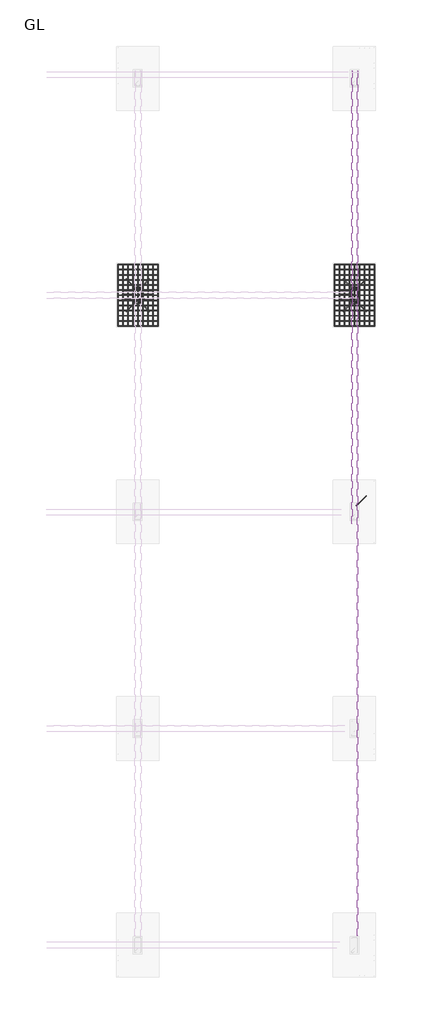
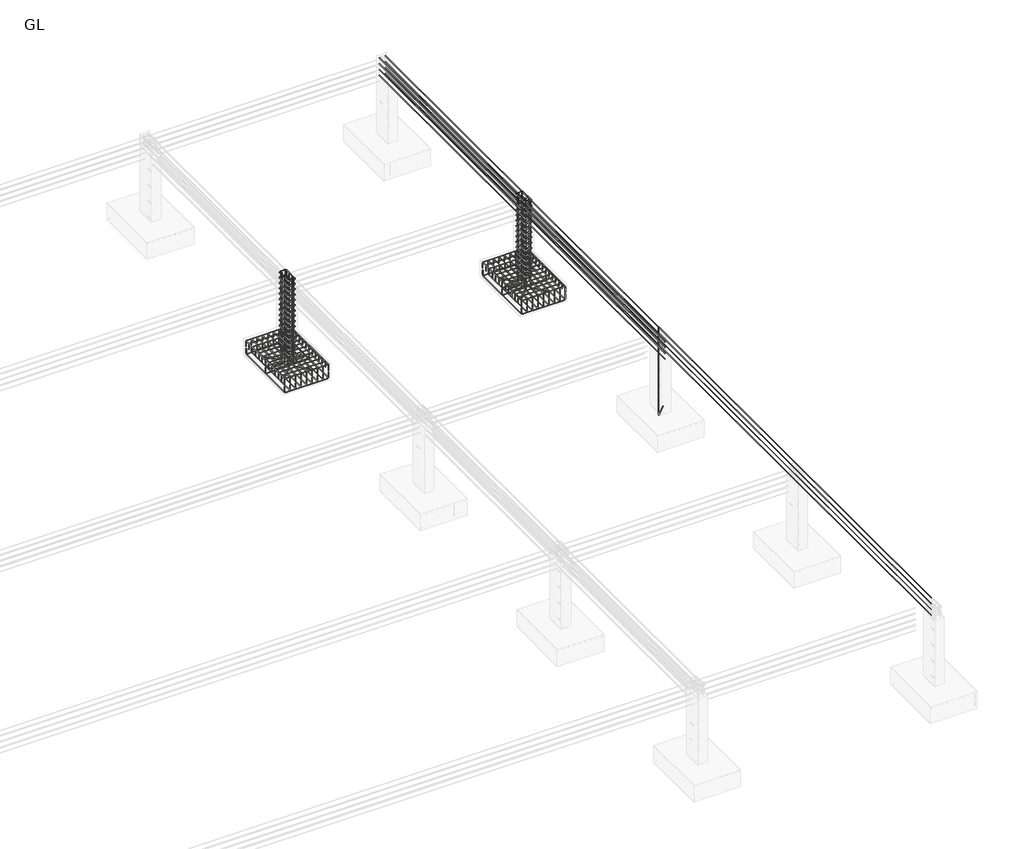
# One storey, part 13 of 16: 24 reinforcing bars.
"""IFC4 building model written with IfcOpenShell, lengths in millimetres."""

from ifc_helpers import new_model, si_unit, point, frame, origin, place, context, project, spatial, polyline, circle_curve, trimmed, segment, composite_curve, source, transform, mapped, element, save
from ifc_brep_helpers import swept_disk

model = new_model("IFC4")

# Units and contexts
model_context = context("Model", 3, world=origin())
ifc_project = project(units=[si_unit("LENGTHUNIT", "METRE", prefix="MILLI")], contexts=[model_context])

# Site, building, storey
site = spatial("IfcSite", under=ifc_project)
building = spatial("IfcBuilding", under=site)
storey = spatial("IfcBuildingStorey", under=building, Name="GL", Elevation=-1829.0)

# Reinforcing bars
placement = place(None, origin())
reinforcing_bar_shape = source(origin(), model_context, "Body", "SolidModel", [
    swept_disk(composite_curve([segment(polyline([(8237.0455621, -1127.1167521, -2089.0), (8237.0455621, -1127.1167521, -2213.0)]), True, "CONTINUOUS"), segment(trimmed(circle_curve(frame((8207.0455621, -1127.1167521, -2213.0), z_axis=(0.0, 1.0, 0.0), x_axis=(30.0, 0.0, 0.0)), 30.0), [point((8237.0455621, -1127.1167521, -2213.0))], [point((8207.0455621, -1127.1167521, -2243.0))], True, "CARTESIAN"), True, "CONTINUOUS"), segment(polyline([(8207.0455621, -1127.1167521, -2243.0), (7139.0455621, -1127.1167521, -2243.0)]), True, "CONTINUOUS"), segment(trimmed(circle_curve(frame((7139.0455621, -1127.1167521, -2213.0), z_axis=(0.0, 1.0, 0.0), x_axis=(0.0, 0.0, -30.0)), 30.0), [point((7139.0455621, -1127.1167521, -2243.0))], [point((7109.0455621, -1127.1167521, -2213.0))], True, "CARTESIAN"), True, "CONTINUOUS"), segment(polyline([(7109.0455621, -1127.1167521, -2213.0), (7109.0455621, -1127.1167521, -2089.0)]), True, "CONTINUOUS")], self_intersect=False), 6.0),
])
element("IfcReinforcingBar", 1, at=placement, inside=storey, context=model_context, shape_type="MappedRepresentation", body=[
    mapped(reinforcing_bar_shape, transform((0.0, 0.0, 0.0), x_axis=(1.0, 0.0, 0.0), y_axis=(0.0, 1.0, 0.0), z_axis=(0.0, 0.0, 1.0))),
    mapped(reinforcing_bar_shape, transform((0.0, -864.0, 0.0), x_axis=(1.0, 0.0, 0.0), y_axis=(0.0, 1.0, 0.0), z_axis=(0.0, 0.0, 1.0))),
    mapped(reinforcing_bar_shape, transform((0.0, -1728.0, 0.0), x_axis=(1.0, 0.0, 0.0), y_axis=(0.0, 1.0, 0.0), z_axis=(0.0, 0.0, 1.0))),
])
reinforcing_bar_2_shape = source(origin(), model_context, "Body", "SolidModel", [
    swept_disk(composite_curve([segment(polyline([(7109.0455621, -1127.1167521, -2022.436678), (7109.0455621, -1127.1167521, -1898.436678)]), True, "CONTINUOUS"), segment(trimmed(circle_curve(frame((7139.0455621, -1127.1167521, -1898.436678), z_axis=(0.0, 1.0, 0.0), x_axis=(-30.0, 0.0, 0.0)), 30.0), [point((7109.0455621, -1127.1167521, -1898.436678))], [point((7139.0455621, -1127.1167521, -1868.436678))], True, "CARTESIAN"), True, "CONTINUOUS"), segment(polyline([(7139.0455621, -1127.1167521, -1868.436678), (8207.0455621, -1127.1167521, -1868.436678)]), True, "CONTINUOUS"), segment(trimmed(circle_curve(frame((8207.0455621, -1127.1167521, -1898.436678), z_axis=(0.0, 1.0, 0.0), x_axis=(0.0, 0.0, 30.0)), 30.0), [point((8207.0455621, -1127.1167521, -1868.436678))], [point((8237.0455621, -1127.1167521, -1898.436678))], True, "CARTESIAN"), True, "CONTINUOUS"), segment(polyline([(8237.0455621, -1127.1167521, -1898.436678), (8237.0455621, -1127.1167521, -2022.436678)]), True, "CONTINUOUS")], self_intersect=False), 6.0),
])
element("IfcReinforcingBar", 2, at=placement, inside=storey, context=model_context, shape_type="MappedRepresentation", body=[
    mapped(reinforcing_bar_2_shape, transform((0.0, 0.0, 0.0), x_axis=(1.0, 0.0, 0.0), y_axis=(0.0, 1.0, 0.0), z_axis=(0.0, 0.0, 1.0))),
    mapped(reinforcing_bar_2_shape, transform((0.0, -144.0, 0.0), x_axis=(1.0, 0.0, 0.0), y_axis=(0.0, 1.0, 0.0), z_axis=(0.0, 0.0, 1.0))),
    mapped(reinforcing_bar_2_shape, transform((0.0, -288.0, 0.0), x_axis=(1.0, 0.0, 0.0), y_axis=(0.0, 1.0, 0.0), z_axis=(0.0, 0.0, 1.0))),
    mapped(reinforcing_bar_2_shape, transform((0.0, -432.0, 0.0), x_axis=(1.0, 0.0, 0.0), y_axis=(0.0, 1.0, 0.0), z_axis=(0.0, 0.0, 1.0))),
    mapped(reinforcing_bar_2_shape, transform((0.0, -576.0, 0.0), x_axis=(1.0, 0.0, 0.0), y_axis=(0.0, 1.0, 0.0), z_axis=(0.0, 0.0, 1.0))),
    mapped(reinforcing_bar_2_shape, transform((0.0, -720.0, 0.0), x_axis=(1.0, 0.0, 0.0), y_axis=(0.0, 1.0, 0.0), z_axis=(0.0, 0.0, 1.0))),
    mapped(reinforcing_bar_2_shape, transform((0.0, -864.0, 0.0), x_axis=(1.0, 0.0, 0.0), y_axis=(0.0, 1.0, 0.0), z_axis=(0.0, 0.0, 1.0))),
    mapped(reinforcing_bar_2_shape, transform((0.0, -1008.0, 0.0), x_axis=(1.0, 0.0, 0.0), y_axis=(0.0, 1.0, 0.0), z_axis=(0.0, 0.0, 1.0))),
    mapped(reinforcing_bar_2_shape, transform((0.0, -1152.0, 0.0), x_axis=(1.0, 0.0, 0.0), y_axis=(0.0, 1.0, 0.0), z_axis=(0.0, 0.0, 1.0))),
    mapped(reinforcing_bar_2_shape, transform((0.0, -1296.0, 0.0), x_axis=(1.0, 0.0, 0.0), y_axis=(0.0, 1.0, 0.0), z_axis=(0.0, 0.0, 1.0))),
    mapped(reinforcing_bar_2_shape, transform((0.0, -1440.0, 0.0), x_axis=(1.0, 0.0, 0.0), y_axis=(0.0, 1.0, 0.0), z_axis=(0.0, 0.0, 1.0))),
    mapped(reinforcing_bar_2_shape, transform((0.0, -1584.0, 0.0), x_axis=(1.0, 0.0, 0.0), y_axis=(0.0, 1.0, 0.0), z_axis=(0.0, 0.0, 1.0))),
    mapped(reinforcing_bar_2_shape, transform((0.0, -1728.0, 0.0), x_axis=(1.0, 0.0, 0.0), y_axis=(0.0, 1.0, 0.0), z_axis=(0.0, 0.0, 1.0))),
])
reinforcing_bar_3_shape = source(origin(), model_context, "Body", "SolidModel", [
    swept_disk(composite_curve([segment(polyline([(7109.0455621, -2855.1167521, -2027.5081232), (7109.0455621, -2855.1167521, -1903.5081232)]), True, "CONTINUOUS"), segment(trimmed(circle_curve(frame((7109.0455621, -2825.1167521, -1903.5081232), z_axis=(-1.0, 0.0, 0.0), x_axis=(0.0, -30.0, 0.0)), 30.0), [point((7109.0455621, -2855.1167521, -1903.5081232))], [point((7109.0455621, -2825.1167521, -1873.5081232))], True, "CARTESIAN"), True, "CONTINUOUS"), segment(polyline([(7109.0455621, -2825.1167521, -1873.5081232), (7109.0455621, -1157.1167521, -1873.5081232)]), True, "CONTINUOUS"), segment(trimmed(circle_curve(frame((7109.0455621, -1157.1167521, -1903.5081232), z_axis=(-1.0, 0.0, 0.0), x_axis=(0.0, 0.0, 30.0)), 30.0), [point((7109.0455621, -1157.1167521, -1873.5081232))], [point((7109.0455621, -1127.1167521, -1903.5081232))], True, "CARTESIAN"), True, "CONTINUOUS"), segment(polyline([(7109.0455621, -1127.1167521, -1903.5081232), (7109.0455621, -1127.1167521, -2027.5081232)]), True, "CONTINUOUS")], self_intersect=False), 6.0),
])
element("IfcReinforcingBar", 3, at=placement, inside=storey, context=model_context, shape_type="MappedRepresentation", body=[
    mapped(reinforcing_bar_3_shape, transform((0.0, 0.0, 0.0), x_axis=(1.0, 0.0, 0.0), y_axis=(0.0, 1.0, 0.0), z_axis=(0.0, 0.0, 1.0))),
    mapped(reinforcing_bar_3_shape, transform((141.0, 0.0, 0.0), x_axis=(1.0, 0.0, 0.0), y_axis=(0.0, 1.0, 0.0), z_axis=(0.0, 0.0, 1.0))),
    mapped(reinforcing_bar_3_shape, transform((282.0, 0.0, 0.0), x_axis=(1.0, 0.0, 0.0), y_axis=(0.0, 1.0, 0.0), z_axis=(0.0, 0.0, 1.0))),
    mapped(reinforcing_bar_3_shape, transform((423.0, 0.0, 0.0), x_axis=(1.0, 0.0, 0.0), y_axis=(0.0, 1.0, 0.0), z_axis=(0.0, 0.0, 1.0))),
    mapped(reinforcing_bar_3_shape, transform((564.0, 0.0, 0.0), x_axis=(1.0, 0.0, 0.0), y_axis=(0.0, 1.0, 0.0), z_axis=(0.0, 0.0, 1.0))),
    mapped(reinforcing_bar_3_shape, transform((705.0, 0.0, 0.0), x_axis=(1.0, 0.0, 0.0), y_axis=(0.0, 1.0, 0.0), z_axis=(0.0, 0.0, 1.0))),
    mapped(reinforcing_bar_3_shape, transform((846.0, 0.0, 0.0), x_axis=(1.0, 0.0, 0.0), y_axis=(0.0, 1.0, 0.0), z_axis=(0.0, 0.0, 1.0))),
    mapped(reinforcing_bar_3_shape, transform((987.0, 0.0, 0.0), x_axis=(1.0, 0.0, 0.0), y_axis=(0.0, 1.0, 0.0), z_axis=(0.0, 0.0, 1.0))),
    mapped(reinforcing_bar_3_shape, transform((1128.0, 0.0, 0.0), x_axis=(1.0, 0.0, 0.0), y_axis=(0.0, 1.0, 0.0), z_axis=(0.0, 0.0, 1.0))),
])
reinforcing_bar_4_shape = source(origin(), model_context, "Body", "SolidModel", [
    swept_disk(composite_curve([segment(polyline([(8237.0455621, -2855.1167521, -2080.6239909), (8237.0455621, -2855.1167521, -2204.6239909)]), True, "CONTINUOUS"), segment(trimmed(circle_curve(frame((8237.0455621, -2825.1167521, -2204.6239909), z_axis=(1.0, 0.0, 0.0), x_axis=(0.0, -30.0, 0.0)), 30.0), [point((8237.0455621, -2855.1167521, -2204.6239909))], [point((8237.0455621, -2825.1167521, -2234.6239909))], True, "CARTESIAN"), True, "CONTINUOUS"), segment(polyline([(8237.0455621, -2825.1167521, -2234.6239909), (8237.0455621, -1170.1421892, -2234.6239909)]), True, "CONTINUOUS"), segment(trimmed(circle_curve(frame((8237.0455621, -1170.1421892, -2204.6239909), z_axis=(1.0, 0.0, 0.0), x_axis=(0.0, 0.0, -30.0)), 30.0), [point((8237.0455621, -1170.1421892, -2234.6239909))], [point((8237.0455621, -1140.1421892, -2204.6239909))], True, "CARTESIAN"), True, "CONTINUOUS"), segment(polyline([(8237.0455621, -1140.1421892, -2204.6239909), (8237.0455621, -1140.1421892, -2080.6239909)]), True, "CONTINUOUS")], self_intersect=False), 6.0),
])
element("IfcReinforcingBar", 4, at=placement, inside=storey, context=model_context, shape_type="MappedRepresentation", body=[
    mapped(reinforcing_bar_4_shape, transform((0.0, 0.0, 0.0), x_axis=(1.0, 0.0, 0.0), y_axis=(0.0, 1.0, 0.0), z_axis=(0.0, 0.0, 1.0))),
    mapped(reinforcing_bar_4_shape, transform((-141.0, 0.0, 0.0), x_axis=(1.0, 0.0, 0.0), y_axis=(0.0, 1.0, 0.0), z_axis=(0.0, 0.0, 1.0))),
    mapped(reinforcing_bar_4_shape, transform((-282.0, 0.0, 0.0), x_axis=(1.0, 0.0, 0.0), y_axis=(0.0, 1.0, 0.0), z_axis=(0.0, 0.0, 1.0))),
    mapped(reinforcing_bar_4_shape, transform((-423.0, 0.0, 0.0), x_axis=(1.0, 0.0, 0.0), y_axis=(0.0, 1.0, 0.0), z_axis=(0.0, 0.0, 1.0))),
    mapped(reinforcing_bar_4_shape, transform((-564.0, 0.0, 0.0), x_axis=(1.0, 0.0, 0.0), y_axis=(0.0, 1.0, 0.0), z_axis=(0.0, 0.0, 1.0))),
    mapped(reinforcing_bar_4_shape, transform((-705.0, 0.0, 0.0), x_axis=(1.0, 0.0, 0.0), y_axis=(0.0, 1.0, 0.0), z_axis=(0.0, 0.0, 1.0))),
    mapped(reinforcing_bar_4_shape, transform((-846.0, 0.0, 0.0), x_axis=(1.0, 0.0, 0.0), y_axis=(0.0, 1.0, 0.0), z_axis=(0.0, 0.0, 1.0))),
    mapped(reinforcing_bar_4_shape, transform((-987.0, 0.0, 0.0), x_axis=(1.0, 0.0, 0.0), y_axis=(0.0, 1.0, 0.0), z_axis=(0.0, 0.0, 1.0))),
    mapped(reinforcing_bar_4_shape, transform((-1128.0, 0.0, 0.0), x_axis=(1.0, 0.0, 0.0), y_axis=(0.0, 1.0, 0.0), z_axis=(0.0, 0.0, 1.0))),
])
reinforcing_bar_5_shape = source(origin(), model_context, "Body", "SolidModel", [
    swept_disk(composite_curve([segment(polyline([(2141.0455621, -1127.1167521, -2089.0), (2141.0455621, -1127.1167521, -2213.0)]), True, "CONTINUOUS"), segment(trimmed(circle_curve(frame((2111.0455621, -1127.1167521, -2213.0), z_axis=(0.0, 1.0, 0.0), x_axis=(30.0, 0.0, 0.0)), 30.0), [point((2141.0455621, -1127.1167521, -2213.0))], [point((2111.0455621, -1127.1167521, -2243.0))], True, "CARTESIAN"), True, "CONTINUOUS"), segment(polyline([(2111.0455621, -1127.1167521, -2243.0), (1043.0455621, -1127.1167521, -2243.0)]), True, "CONTINUOUS"), segment(trimmed(circle_curve(frame((1043.0455621, -1127.1167521, -2213.0), z_axis=(0.0, 1.0, 0.0), x_axis=(0.0, 0.0, -30.0)), 30.0), [point((1043.0455621, -1127.1167521, -2243.0))], [point((1013.0455621, -1127.1167521, -2213.0))], True, "CARTESIAN"), True, "CONTINUOUS"), segment(polyline([(1013.0455621, -1127.1167521, -2213.0), (1013.0455621, -1127.1167521, -2089.0)]), True, "CONTINUOUS")], self_intersect=False), 6.0),
])
element("IfcReinforcingBar", 5, at=placement, inside=storey, context=model_context, shape_type="MappedRepresentation", body=[
    mapped(reinforcing_bar_5_shape, transform((0.0, 0.0, 0.0), x_axis=(1.0, 0.0, 0.0), y_axis=(0.0, 1.0, 0.0), z_axis=(0.0, 0.0, 1.0))),
    mapped(reinforcing_bar_5_shape, transform((0.0, -864.0, 0.0), x_axis=(1.0, 0.0, 0.0), y_axis=(0.0, 1.0, 0.0), z_axis=(0.0, 0.0, 1.0))),
    mapped(reinforcing_bar_5_shape, transform((0.0, -1728.0, 0.0), x_axis=(1.0, 0.0, 0.0), y_axis=(0.0, 1.0, 0.0), z_axis=(0.0, 0.0, 1.0))),
])
reinforcing_bar_6_shape = source(origin(), model_context, "Body", "SolidModel", [
    swept_disk(composite_curve([segment(polyline([(1013.0455621, -1127.1167521, -2022.436678), (1013.0455621, -1127.1167521, -1898.436678)]), True, "CONTINUOUS"), segment(trimmed(circle_curve(frame((1043.0455621, -1127.1167521, -1898.436678), z_axis=(0.0, 1.0, 0.0), x_axis=(-30.000000000000114, 0.0, 0.0)), 30.0), [point((1013.0455621, -1127.1167521, -1898.436678))], [point((1043.0455621, -1127.1167521, -1868.436678))], True, "CARTESIAN"), True, "CONTINUOUS"), segment(polyline([(1043.0455621, -1127.1167521, -1868.436678), (2111.0455621, -1127.1167521, -1868.436678)]), True, "CONTINUOUS"), segment(trimmed(circle_curve(frame((2111.0455621, -1127.1167521, -1898.436678), z_axis=(0.0, 1.0, 0.0), x_axis=(0.0, 0.0, 30.0)), 30.0), [point((2111.0455621, -1127.1167521, -1868.436678))], [point((2141.0455621, -1127.1167521, -1898.436678))], True, "CARTESIAN"), True, "CONTINUOUS"), segment(polyline([(2141.0455621, -1127.1167521, -1898.436678), (2141.0455621, -1127.1167521, -2022.436678)]), True, "CONTINUOUS")], self_intersect=False), 6.0),
])
element("IfcReinforcingBar", 6, at=placement, inside=storey, context=model_context, shape_type="MappedRepresentation", body=[
    mapped(reinforcing_bar_6_shape, transform((0.0, 0.0, 0.0), x_axis=(1.0, 0.0, 0.0), y_axis=(0.0, 1.0, 0.0), z_axis=(0.0, 0.0, 1.0))),
    mapped(reinforcing_bar_6_shape, transform((0.0, -144.0, 0.0), x_axis=(1.0, 0.0, 0.0), y_axis=(0.0, 1.0, 0.0), z_axis=(0.0, 0.0, 1.0))),
    mapped(reinforcing_bar_6_shape, transform((0.0, -288.0, 0.0), x_axis=(1.0, 0.0, 0.0), y_axis=(0.0, 1.0, 0.0), z_axis=(0.0, 0.0, 1.0))),
    mapped(reinforcing_bar_6_shape, transform((0.0, -432.0, 0.0), x_axis=(1.0, 0.0, 0.0), y_axis=(0.0, 1.0, 0.0), z_axis=(0.0, 0.0, 1.0))),
    mapped(reinforcing_bar_6_shape, transform((0.0, -576.0, 0.0), x_axis=(1.0, 0.0, 0.0), y_axis=(0.0, 1.0, 0.0), z_axis=(0.0, 0.0, 1.0))),
    mapped(reinforcing_bar_6_shape, transform((0.0, -720.0, 0.0), x_axis=(1.0, 0.0, 0.0), y_axis=(0.0, 1.0, 0.0), z_axis=(0.0, 0.0, 1.0))),
    mapped(reinforcing_bar_6_shape, transform((0.0, -864.0, 0.0), x_axis=(1.0, 0.0, 0.0), y_axis=(0.0, 1.0, 0.0), z_axis=(0.0, 0.0, 1.0))),
    mapped(reinforcing_bar_6_shape, transform((0.0, -1008.0, 0.0), x_axis=(1.0, 0.0, 0.0), y_axis=(0.0, 1.0, 0.0), z_axis=(0.0, 0.0, 1.0))),
    mapped(reinforcing_bar_6_shape, transform((0.0, -1152.0, 0.0), x_axis=(1.0, 0.0, 0.0), y_axis=(0.0, 1.0, 0.0), z_axis=(0.0, 0.0, 1.0))),
    mapped(reinforcing_bar_6_shape, transform((0.0, -1296.0, 0.0), x_axis=(1.0, 0.0, 0.0), y_axis=(0.0, 1.0, 0.0), z_axis=(0.0, 0.0, 1.0))),
    mapped(reinforcing_bar_6_shape, transform((0.0, -1440.0, 0.0), x_axis=(1.0, 0.0, 0.0), y_axis=(0.0, 1.0, 0.0), z_axis=(0.0, 0.0, 1.0))),
    mapped(reinforcing_bar_6_shape, transform((0.0, -1584.0, 0.0), x_axis=(1.0, 0.0, 0.0), y_axis=(0.0, 1.0, 0.0), z_axis=(0.0, 0.0, 1.0))),
    mapped(reinforcing_bar_6_shape, transform((0.0, -1728.0, 0.0), x_axis=(1.0, 0.0, 0.0), y_axis=(0.0, 1.0, 0.0), z_axis=(0.0, 0.0, 1.0))),
])
reinforcing_bar_7_shape = source(origin(), model_context, "Body", "SolidModel", [
    swept_disk(composite_curve([segment(polyline([(1013.0455621, -2855.1167521, -2027.5081232), (1013.0455621, -2855.1167521, -1903.5081232)]), True, "CONTINUOUS"), segment(trimmed(circle_curve(frame((1013.0455621, -2825.1167521, -1903.5081232), z_axis=(-1.0, 0.0, 0.0), x_axis=(0.0, -30.0, 0.0)), 30.0), [point((1013.0455621, -2855.1167521, -1903.5081232))], [point((1013.0455621, -2825.1167521, -1873.5081232))], True, "CARTESIAN"), True, "CONTINUOUS"), segment(polyline([(1013.0455621, -2825.1167521, -1873.5081232), (1013.0455621, -1157.1167521, -1873.5081232)]), True, "CONTINUOUS"), segment(trimmed(circle_curve(frame((1013.0455621, -1157.1167521, -1903.5081232), z_axis=(-1.0, 0.0, 0.0), x_axis=(0.0, 0.0, 30.0)), 30.0), [point((1013.0455621, -1157.1167521, -1873.5081232))], [point((1013.0455621, -1127.1167521, -1903.5081232))], True, "CARTESIAN"), True, "CONTINUOUS"), segment(polyline([(1013.0455621, -1127.1167521, -1903.5081232), (1013.0455621, -1127.1167521, -2027.5081232)]), True, "CONTINUOUS")], self_intersect=False), 6.0),
])
element("IfcReinforcingBar", 7, at=placement, inside=storey, context=model_context, shape_type="MappedRepresentation", body=[
    mapped(reinforcing_bar_7_shape, transform((0.0, 0.0, 0.0), x_axis=(1.0, 0.0, 0.0), y_axis=(0.0, 1.0, 0.0), z_axis=(0.0, 0.0, 1.0))),
    mapped(reinforcing_bar_7_shape, transform((141.0, 0.0, 0.0), x_axis=(1.0, 0.0, 0.0), y_axis=(0.0, 1.0, 0.0), z_axis=(0.0, 0.0, 1.0))),
    mapped(reinforcing_bar_7_shape, transform((282.0, 0.0, 0.0), x_axis=(1.0, 0.0, 0.0), y_axis=(0.0, 1.0, 0.0), z_axis=(0.0, 0.0, 1.0))),
    mapped(reinforcing_bar_7_shape, transform((423.0, 0.0, 0.0), x_axis=(1.0, 0.0, 0.0), y_axis=(0.0, 1.0, 0.0), z_axis=(0.0, 0.0, 1.0))),
    mapped(reinforcing_bar_7_shape, transform((564.0, 0.0, 0.0), x_axis=(1.0, 0.0, 0.0), y_axis=(0.0, 1.0, 0.0), z_axis=(0.0, 0.0, 1.0))),
    mapped(reinforcing_bar_7_shape, transform((705.0, 0.0, 0.0), x_axis=(1.0, 0.0, 0.0), y_axis=(0.0, 1.0, 0.0), z_axis=(0.0, 0.0, 1.0))),
    mapped(reinforcing_bar_7_shape, transform((846.0, 0.0, 0.0), x_axis=(1.0, 0.0, 0.0), y_axis=(0.0, 1.0, 0.0), z_axis=(0.0, 0.0, 1.0))),
    mapped(reinforcing_bar_7_shape, transform((987.0, 0.0, 0.0), x_axis=(1.0, 0.0, 0.0), y_axis=(0.0, 1.0, 0.0), z_axis=(0.0, 0.0, 1.0))),
    mapped(reinforcing_bar_7_shape, transform((1128.0, 0.0, 0.0), x_axis=(1.0, 0.0, 0.0), y_axis=(0.0, 1.0, 0.0), z_axis=(0.0, 0.0, 1.0))),
])
reinforcing_bar_8_shape = source(origin(), model_context, "Body", "SolidModel", [
    swept_disk(composite_curve([segment(polyline([(2141.0455621, -2855.1167521, -2080.6239909), (2141.0455621, -2855.1167521, -2204.6239909)]), True, "CONTINUOUS"), segment(trimmed(circle_curve(frame((2141.0455621, -2825.1167521, -2204.6239909), z_axis=(1.0, 0.0, 0.0), x_axis=(0.0, -30.0, 0.0)), 30.0), [point((2141.0455621, -2855.1167521, -2204.6239909))], [point((2141.0455621, -2825.1167521, -2234.6239909))], True, "CARTESIAN"), True, "CONTINUOUS"), segment(polyline([(2141.0455621, -2825.1167521, -2234.6239909), (2141.0455621, -1170.1421892, -2234.6239909)]), True, "CONTINUOUS"), segment(trimmed(circle_curve(frame((2141.0455621, -1170.1421892, -2204.6239909), z_axis=(1.0, 0.0, 0.0), x_axis=(0.0, 0.0, -30.0)), 30.0), [point((2141.0455621, -1170.1421892, -2234.6239909))], [point((2141.0455621, -1140.1421892, -2204.6239909))], True, "CARTESIAN"), True, "CONTINUOUS"), segment(polyline([(2141.0455621, -1140.1421892, -2204.6239909), (2141.0455621, -1140.1421892, -2080.6239909)]), True, "CONTINUOUS")], self_intersect=False), 6.0),
])
element("IfcReinforcingBar", 8, at=placement, inside=storey, context=model_context, shape_type="MappedRepresentation", body=[
    mapped(reinforcing_bar_8_shape, transform((0.0, 0.0, 0.0), x_axis=(1.0, 0.0, 0.0), y_axis=(0.0, 1.0, 0.0), z_axis=(0.0, 0.0, 1.0))),
    mapped(reinforcing_bar_8_shape, transform((-141.0, 0.0, 0.0), x_axis=(1.0, 0.0, 0.0), y_axis=(0.0, 1.0, 0.0), z_axis=(0.0, 0.0, 1.0))),
    mapped(reinforcing_bar_8_shape, transform((-282.0, 0.0, 0.0), x_axis=(1.0, 0.0, 0.0), y_axis=(0.0, 1.0, 0.0), z_axis=(0.0, 0.0, 1.0))),
    mapped(reinforcing_bar_8_shape, transform((-423.0, 0.0, 0.0), x_axis=(1.0, 0.0, 0.0), y_axis=(0.0, 1.0, 0.0), z_axis=(0.0, 0.0, 1.0))),
    mapped(reinforcing_bar_8_shape, transform((-564.0, 0.0, 0.0), x_axis=(1.0, 0.0, 0.0), y_axis=(0.0, 1.0, 0.0), z_axis=(0.0, 0.0, 1.0))),
    mapped(reinforcing_bar_8_shape, transform((-705.0, 0.0, 0.0), x_axis=(1.0, 0.0, 0.0), y_axis=(0.0, 1.0, 0.0), z_axis=(0.0, 0.0, 1.0))),
    mapped(reinforcing_bar_8_shape, transform((-846.0, 0.0, 0.0), x_axis=(1.0, 0.0, 0.0), y_axis=(0.0, 1.0, 0.0), z_axis=(0.0, 0.0, 1.0))),
    mapped(reinforcing_bar_8_shape, transform((-987.0, 0.0, 0.0), x_axis=(1.0, 0.0, 0.0), y_axis=(0.0, 1.0, 0.0), z_axis=(0.0, 0.0, 1.0))),
    mapped(reinforcing_bar_8_shape, transform((-1128.0, 0.0, 0.0), x_axis=(1.0, 0.0, 0.0), y_axis=(0.0, 1.0, 0.0), z_axis=(0.0, 0.0, 1.0))),
])
element("IfcReinforcingBar", 9, at=placement, inside=storey, context=model_context, shape_type="SolidModel", body=[
    swept_disk(composite_curve([segment(polyline([(7730.1553473, -7902.1692603, 241.0), (7730.1553473, -7902.1692603, -2129.0)]), True, "CONTINUOUS"), segment(trimmed(circle_curve(frame((7751.3685508, -7880.9560568, -2129.0), z_axis=(0.7071067811865157, -0.7071067811865794, 0.0), x_axis=(-21.21320349999951, -21.213203500000418, 0.0)), 30.0), [point((7730.1553473, -7902.1692603, -2129.0))], [point((7751.3685508, -7880.9560568, -2159.0))], True, "CARTESIAN"), True, "CONTINUOUS"), segment(polyline([(7751.3685508, -7880.9560568, -2159.0), (7998.8559242, -7633.4686834, -2159.0)]), True, "CONTINUOUS")], self_intersect=False), 6.0),
])
reinforcing_bar_9_shape = source(origin(), model_context, "Body", "SolidModel", [
    swept_disk(composite_curve([segment(polyline([(1584.5135995, -2066.2223078, -1793.0), (1496.8323586, -2153.9035486, -1793.0)]), True, "CONTINUOUS"), segment(trimmed(circle_curve(frame((1518.0455621, -2175.1167521, -1793.0), z_axis=(0.0, 0.0, 1.0), x_axis=(-21.21320350000019, 21.213203500000418, 0.0)), 30.0), [point((1496.8323586, -2153.9035486, -1793.0))], [point((1518.0455621, -2205.1167521, -1793.0))], True, "CARTESIAN"), True, "CONTINUOUS"), segment(polyline([(1518.0455621, -2205.1167521, -1793.0), (1636.0455621, -2205.1167521, -1793.0)]), True, "CONTINUOUS"), segment(trimmed(circle_curve(frame((1636.0455621, -2175.1167521, -1793.0), z_axis=(0.0, 0.0, 1.0), x_axis=(0.0, -30.0, 0.0)), 30.0), [point((1636.0455621, -2205.1167521, -1793.0))], [point((1666.0455621, -2175.1167521, -1793.0))], True, "CARTESIAN"), True, "CONTINUOUS"), segment(polyline([(1666.0455621, -2175.1167521, -1793.0), (1666.0455621, -1807.1167521, -1793.0)]), True, "CONTINUOUS"), segment(trimmed(circle_curve(frame((1636.1135038, -1807.1167521, -1795.0178916), z_axis=(-0.06726305234213417, 0.0, 0.9977352764083365), x_axis=(29.932058300000108, 0.0, 2.0178915999999845)), 30.0), [point((1666.0455621, -1807.1167521, -1793.0))], [point((1636.1135038, -1777.1167521, -1795.0178916))], True, "CARTESIAN"), True, "CONTINUOUS"), segment(polyline([(1636.1135038, -1777.1167521, -1795.0178916), (1517.9776204, -1777.1167521, -1802.9821084)]), True, "CONTINUOUS"), segment(trimmed(circle_curve(frame((1517.9776204, -1807.1167521, -1802.9821084), z_axis=(-0.06726305234213417, 0.0, 0.9977352764083365), x_axis=(0.0, 30.0, 0.0)), 30.0), [point((1517.9776204, -1777.1167521, -1802.9821084))], [point((1488.0455621, -1807.1167521, -1805.0))], True, "CARTESIAN"), True, "CONTINUOUS"), segment(polyline([(1488.0455621, -1807.1167521, -1805.0), (1488.0455621, -2175.1167521, -1805.0)]), True, "CONTINUOUS"), segment(trimmed(circle_curve(frame((1518.0455621, -2175.1167521, -1805.0), z_axis=(0.0, 0.0, 1.0), x_axis=(-30.0, 0.0, 0.0)), 30.0), [point((1488.0455621, -2175.1167521, -1805.0))], [point((1539.2587655, -2196.3299555, -1805.0))], True, "CARTESIAN"), True, "CONTINUOUS"), segment(polyline([(1539.2587655, -2196.3299555, -1805.0), (1626.9400064, -2108.6487146, -1805.0)]), True, "CONTINUOUS")], self_intersect=False), 6.0),
])
element("IfcReinforcingBar", 10, at=placement, inside=storey, context=model_context, shape_type="MappedRepresentation", body=[
    mapped(reinforcing_bar_9_shape, transform((0.0, 0.0, 0.0), x_axis=(1.0, 0.0, 0.0), y_axis=(0.0, 1.0, 0.0), z_axis=(0.0, 0.0, 1.0))),
    mapped(reinforcing_bar_9_shape, transform((0.0, 0.0, 144.8571429), x_axis=(1.0, 0.0, 0.0), y_axis=(0.0, 1.0, 0.0), z_axis=(0.0, 0.0, 1.0))),
    mapped(reinforcing_bar_9_shape, transform((0.0, 0.0, 289.7142857), x_axis=(1.0, 0.0, 0.0), y_axis=(0.0, 1.0, 0.0), z_axis=(0.0, 0.0, 1.0))),
    mapped(reinforcing_bar_9_shape, transform((0.0, 0.0, 434.5714286), x_axis=(1.0, 0.0, 0.0), y_axis=(0.0, 1.0, 0.0), z_axis=(0.0, 0.0, 1.0))),
    mapped(reinforcing_bar_9_shape, transform((0.0, 0.0, 579.4285714), x_axis=(1.0, 0.0, 0.0), y_axis=(0.0, 1.0, 0.0), z_axis=(0.0, 0.0, 1.0))),
    mapped(reinforcing_bar_9_shape, transform((0.0, 0.0, 724.2857143), x_axis=(1.0, 0.0, 0.0), y_axis=(0.0, 1.0, 0.0), z_axis=(0.0, 0.0, 1.0))),
    mapped(reinforcing_bar_9_shape, transform((0.0, 0.0, 869.1428571), x_axis=(1.0, 0.0, 0.0), y_axis=(0.0, 1.0, 0.0), z_axis=(0.0, 0.0, 1.0))),
    mapped(reinforcing_bar_9_shape, transform((0.0, 0.0, 1014.0), x_axis=(1.0, 0.0, 0.0), y_axis=(0.0, 1.0, 0.0), z_axis=(0.0, 0.0, 1.0))),
    mapped(reinforcing_bar_9_shape, transform((0.0, 0.0, 1158.8571429), x_axis=(1.0, 0.0, 0.0), y_axis=(0.0, 1.0, 0.0), z_axis=(0.0, 0.0, 1.0))),
    mapped(reinforcing_bar_9_shape, transform((0.0, 0.0, 1303.7142857), x_axis=(1.0, 0.0, 0.0), y_axis=(0.0, 1.0, 0.0), z_axis=(0.0, 0.0, 1.0))),
    mapped(reinforcing_bar_9_shape, transform((0.0, 0.0, 1448.5714286), x_axis=(1.0, 0.0, 0.0), y_axis=(0.0, 1.0, 0.0), z_axis=(0.0, 0.0, 1.0))),
    mapped(reinforcing_bar_9_shape, transform((0.0, 0.0, 1593.4285714), x_axis=(1.0, 0.0, 0.0), y_axis=(0.0, 1.0, 0.0), z_axis=(0.0, 0.0, 1.0))),
    mapped(reinforcing_bar_9_shape, transform((0.0, 0.0, 1738.2857143), x_axis=(1.0, 0.0, 0.0), y_axis=(0.0, 1.0, 0.0), z_axis=(0.0, 0.0, 1.0))),
    mapped(reinforcing_bar_9_shape, transform((0.0, 0.0, 1883.1428571), x_axis=(1.0, 0.0, 0.0), y_axis=(0.0, 1.0, 0.0), z_axis=(0.0, 0.0, 1.0))),
    mapped(reinforcing_bar_9_shape, transform((0.0, 0.0, 2028.0), x_axis=(1.0, 0.0, 0.0), y_axis=(0.0, 1.0, 0.0), z_axis=(0.0, 0.0, 1.0))),
])
element("IfcReinforcingBar", 11, at=placement, inside=storey, context=model_context, shape_type="SolidModel", body=[
    swept_disk(composite_curve([segment(polyline([(1519.9357768, -2176.0642439, 241.0), (1519.9357768, -2176.0642439, -2129.0)]), True, "CONTINUOUS"), segment(trimmed(circle_curve(frame((1498.7225734, -2197.2774473, -2129.0), z_axis=(-0.7071067811865187, 0.7071067811865764, 0.0), x_axis=(21.213203399999884, 21.21320340000011, 0.0)), 30.0), [point((1519.9357768, -2176.0642439, -2129.0))], [point((1498.7225734, -2197.2774473, -2159.0))], True, "CARTESIAN"), True, "CONTINUOUS"), segment(polyline([(1498.7225734, -2197.2774473, -2159.0), (1251.2352, -2444.7648207, -2159.0)]), True, "CONTINUOUS")], self_intersect=False), 6.0),
])
element("IfcReinforcingBar", 12, at=placement, inside=storey, context=model_context, shape_type="SolidModel", body=[
    swept_disk(composite_curve([segment(polyline([(1519.9357768, -1806.1692603, 241.0), (1519.9357768, -1806.1692603, -2129.0)]), True, "CONTINUOUS"), segment(trimmed(circle_curve(frame((1498.7225734, -1784.9560568, -2129.0), z_axis=(0.7071067811865218, 0.7071067811865733, 0.0), x_axis=(21.213203399999884, -21.213203499999963, 0.0)), 30.0), [point((1519.9357768, -1806.1692603, -2129.0))], [point((1498.7225734, -1784.9560568, -2159.0))], True, "CARTESIAN"), True, "CONTINUOUS"), segment(polyline([(1498.7225734, -1784.9560568, -2159.0), (1251.2352, -1537.4686834, -2159.0)]), True, "CONTINUOUS")], self_intersect=False), 6.0),
])
element("IfcReinforcingBar", 13, at=placement, inside=storey, context=model_context, shape_type="SolidModel", body=[
    swept_disk(composite_curve([segment(polyline([(1634.1553473, -2176.0642439, 241.0), (1634.1553473, -2176.0642439, -2129.0)]), True, "CONTINUOUS"), segment(trimmed(circle_curve(frame((1655.3685508, -2197.2774473, -2129.0), z_axis=(-0.7071067811865248, -0.7071067811865703, 0.0), x_axis=(-21.21320350000019, 21.21320340000011, 0.0)), 30.0), [point((1634.1553473, -2176.0642439, -2129.0))], [point((1655.3685508, -2197.2774473, -2159.0))], True, "CARTESIAN"), True, "CONTINUOUS"), segment(polyline([(1655.3685508, -2197.2774473, -2159.0), (1902.8559242, -2444.7648207, -2159.0)]), True, "CONTINUOUS")], self_intersect=False), 6.0),
])
element("IfcReinforcingBar", 14, at=placement, inside=storey, context=model_context, shape_type="SolidModel", body=[
    swept_disk(composite_curve([segment(polyline([(1634.1553473, -1806.1692603, 241.0), (1634.1553473, -1806.1692603, -2129.0)]), True, "CONTINUOUS"), segment(trimmed(circle_curve(frame((1655.3685508, -1784.9560568, -2129.0), z_axis=(0.7071067811865157, -0.7071067811865794, 0.0), x_axis=(-21.21320350000019, -21.213203499999963, 0.0)), 30.0), [point((1634.1553473, -1806.1692603, -2129.0))], [point((1655.3685508, -1784.9560568, -2159.0))], True, "CARTESIAN"), True, "CONTINUOUS"), segment(polyline([(1655.3685508, -1784.9560568, -2159.0), (1902.8559242, -1537.4686834, -2159.0)]), True, "CONTINUOUS")], self_intersect=False), 6.0),
])
reinforcing_bar_10_shape = source(origin(), model_context, "Body", "SolidModel", [
    swept_disk(composite_curve([segment(polyline([(1519.9357768, -2098.9117405, 241.0), (1519.9357768, -2098.9117405, -2129.0)]), True, "CONTINUOUS"), segment(trimmed(circle_curve(frame((1489.9357768, -2098.9117405, -2129.0), z_axis=(0.0, 1.0, 0.0), x_axis=(30.0, 0.0, 0.0)), 30.0), [point((1519.9357768, -2098.9117405, -2129.0))], [point((1489.9357768, -2098.9117405, -2159.0))], True, "CARTESIAN"), True, "CONTINUOUS"), segment(polyline([(1489.9357768, -2098.9117405, -2159.0), (1139.9357768, -2098.9117405, -2159.0)]), True, "CONTINUOUS")], self_intersect=False), 6.0),
])
element("IfcReinforcingBar", 15, at=placement, inside=storey, context=model_context, shape_type="MappedRepresentation", body=[
    mapped(reinforcing_bar_10_shape, transform((0.0, 0.0, 0.0), x_axis=(1.0, 0.0, 0.0), y_axis=(0.0, 1.0, 0.0), z_axis=(0.0, 0.0, 1.0))),
    mapped(reinforcing_bar_10_shape, transform((0.0, 123.5823926, 0.0), x_axis=(1.0, 0.0, 0.0), y_axis=(0.0, 1.0, 0.0), z_axis=(0.0, 0.0, 1.0))),
    mapped(reinforcing_bar_10_shape, transform((0.0, 247.1647853, 0.0), x_axis=(1.0, 0.0, 0.0), y_axis=(0.0, 1.0, 0.0), z_axis=(0.0, 0.0, 1.0))),
])
reinforcing_bar_11_shape = source(origin(), model_context, "Body", "SolidModel", [
    swept_disk(composite_curve([segment(polyline([(1634.1553473, -2098.9117405, 241.0), (1634.1553473, -2098.9117405, -2129.0)]), True, "CONTINUOUS"), segment(trimmed(circle_curve(frame((1664.1553473, -2098.9117405, -2129.0), z_axis=(0.0, -1.0, 0.0), x_axis=(-30.0, 0.0, 0.0)), 30.0), [point((1634.1553473, -2098.9117405, -2129.0))], [point((1664.1553473, -2098.9117405, -2159.0))], True, "CARTESIAN"), True, "CONTINUOUS"), segment(polyline([(1664.1553473, -2098.9117405, -2159.0), (2014.1553473, -2098.9117405, -2159.0)]), True, "CONTINUOUS")], self_intersect=False), 6.0),
])
element("IfcReinforcingBar", 16, at=placement, inside=storey, context=model_context, shape_type="MappedRepresentation", body=[
    mapped(reinforcing_bar_11_shape, transform((0.0, 0.0, 0.0), x_axis=(1.0, 0.0, 0.0), y_axis=(0.0, 1.0, 0.0), z_axis=(0.0, 0.0, 1.0))),
    mapped(reinforcing_bar_11_shape, transform((0.0, 123.5823926, 0.0), x_axis=(1.0, 0.0, 0.0), y_axis=(0.0, 1.0, 0.0), z_axis=(0.0, 0.0, 1.0))),
    mapped(reinforcing_bar_11_shape, transform((0.0, 247.1647853, 0.0), x_axis=(1.0, 0.0, 0.0), y_axis=(0.0, 1.0, 0.0), z_axis=(0.0, 0.0, 1.0))),
])
reinforcing_bar_12_shape = source(origin(), model_context, "Body", "SolidModel", [
    swept_disk(composite_curve([segment(polyline([(7680.5135995, -2066.2223078, -1793.0), (7592.8323586, -2153.9035486, -1793.0)]), True, "CONTINUOUS"), segment(trimmed(circle_curve(frame((7614.0455621, -2175.1167521, -1793.0), z_axis=(0.0, 0.0, 1.0), x_axis=(-21.213203500000418, 21.213203500000418, 0.0)), 30.0), [point((7592.8323586, -2153.9035486, -1793.0))], [point((7614.0455621, -2205.1167521, -1793.0))], True, "CARTESIAN"), True, "CONTINUOUS"), segment(polyline([(7614.0455621, -2205.1167521, -1793.0), (7732.0455621, -2205.1167521, -1793.0)]), True, "CONTINUOUS"), segment(trimmed(circle_curve(frame((7732.0455621, -2175.1167521, -1793.0), z_axis=(0.0, 0.0, 1.0), x_axis=(0.0, -30.0, 0.0)), 30.0), [point((7732.0455621, -2205.1167521, -1793.0))], [point((7762.0455621, -2175.1167521, -1793.0))], True, "CARTESIAN"), True, "CONTINUOUS"), segment(polyline([(7762.0455621, -2175.1167521, -1793.0), (7762.0455621, -1807.1167521, -1793.0)]), True, "CONTINUOUS"), segment(trimmed(circle_curve(frame((7732.1135038, -1807.1167521, -1795.0178916), z_axis=(-0.06726305234213417, 0.0, 0.9977352764083365), x_axis=(29.93205829999988, 0.0, 2.0178915999999845)), 30.0), [point((7762.0455621, -1807.1167521, -1793.0))], [point((7732.1135038, -1777.1167521, -1795.0178916))], True, "CARTESIAN"), True, "CONTINUOUS"), segment(polyline([(7732.1135038, -1777.1167521, -1795.0178916), (7613.9776204, -1777.1167521, -1802.9821084)]), True, "CONTINUOUS"), segment(trimmed(circle_curve(frame((7613.9776204, -1807.1167521, -1802.9821084), z_axis=(-0.06726305234213417, 0.0, 0.9977352764083365), x_axis=(0.0, 30.0, 0.0)), 30.0), [point((7613.9776204, -1777.1167521, -1802.9821084))], [point((7584.0455621, -1807.1167521, -1805.0))], True, "CARTESIAN"), True, "CONTINUOUS"), segment(polyline([(7584.0455621, -1807.1167521, -1805.0), (7584.0455621, -2175.1167521, -1805.0)]), True, "CONTINUOUS"), segment(trimmed(circle_curve(frame((7614.0455621, -2175.1167521, -1805.0), z_axis=(0.0, 0.0, 1.0), x_axis=(-30.0, 0.0, 0.0)), 30.0), [point((7584.0455621, -2175.1167521, -1805.0))], [point((7635.2587655, -2196.3299555, -1805.0))], True, "CARTESIAN"), True, "CONTINUOUS"), segment(polyline([(7635.2587655, -2196.3299555, -1805.0), (7722.9400064, -2108.6487146, -1805.0)]), True, "CONTINUOUS")], self_intersect=False), 6.0),
])
element("IfcReinforcingBar", 17, at=placement, inside=storey, context=model_context, shape_type="MappedRepresentation", body=[
    mapped(reinforcing_bar_12_shape, transform((0.0, 0.0, 0.0), x_axis=(1.0, 0.0, 0.0), y_axis=(0.0, 1.0, 0.0), z_axis=(0.0, 0.0, 1.0))),
    mapped(reinforcing_bar_12_shape, transform((0.0, 0.0, 144.8571429), x_axis=(1.0, 0.0, 0.0), y_axis=(0.0, 1.0, 0.0), z_axis=(0.0, 0.0, 1.0))),
    mapped(reinforcing_bar_12_shape, transform((0.0, 0.0, 289.7142857), x_axis=(1.0, 0.0, 0.0), y_axis=(0.0, 1.0, 0.0), z_axis=(0.0, 0.0, 1.0))),
    mapped(reinforcing_bar_12_shape, transform((0.0, 0.0, 434.5714286), x_axis=(1.0, 0.0, 0.0), y_axis=(0.0, 1.0, 0.0), z_axis=(0.0, 0.0, 1.0))),
    mapped(reinforcing_bar_12_shape, transform((0.0, 0.0, 579.4285714), x_axis=(1.0, 0.0, 0.0), y_axis=(0.0, 1.0, 0.0), z_axis=(0.0, 0.0, 1.0))),
    mapped(reinforcing_bar_12_shape, transform((0.0, 0.0, 724.2857143), x_axis=(1.0, 0.0, 0.0), y_axis=(0.0, 1.0, 0.0), z_axis=(0.0, 0.0, 1.0))),
    mapped(reinforcing_bar_12_shape, transform((0.0, 0.0, 869.1428571), x_axis=(1.0, 0.0, 0.0), y_axis=(0.0, 1.0, 0.0), z_axis=(0.0, 0.0, 1.0))),
    mapped(reinforcing_bar_12_shape, transform((0.0, 0.0, 1014.0), x_axis=(1.0, 0.0, 0.0), y_axis=(0.0, 1.0, 0.0), z_axis=(0.0, 0.0, 1.0))),
    mapped(reinforcing_bar_12_shape, transform((0.0, 0.0, 1158.8571429), x_axis=(1.0, 0.0, 0.0), y_axis=(0.0, 1.0, 0.0), z_axis=(0.0, 0.0, 1.0))),
    mapped(reinforcing_bar_12_shape, transform((0.0, 0.0, 1303.7142857), x_axis=(1.0, 0.0, 0.0), y_axis=(0.0, 1.0, 0.0), z_axis=(0.0, 0.0, 1.0))),
    mapped(reinforcing_bar_12_shape, transform((0.0, 0.0, 1448.5714286), x_axis=(1.0, 0.0, 0.0), y_axis=(0.0, 1.0, 0.0), z_axis=(0.0, 0.0, 1.0))),
    mapped(reinforcing_bar_12_shape, transform((0.0, 0.0, 1593.4285714), x_axis=(1.0, 0.0, 0.0), y_axis=(0.0, 1.0, 0.0), z_axis=(0.0, 0.0, 1.0))),
    mapped(reinforcing_bar_12_shape, transform((0.0, 0.0, 1738.2857143), x_axis=(1.0, 0.0, 0.0), y_axis=(0.0, 1.0, 0.0), z_axis=(0.0, 0.0, 1.0))),
    mapped(reinforcing_bar_12_shape, transform((0.0, 0.0, 1883.1428571), x_axis=(1.0, 0.0, 0.0), y_axis=(0.0, 1.0, 0.0), z_axis=(0.0, 0.0, 1.0))),
    mapped(reinforcing_bar_12_shape, transform((0.0, 0.0, 2028.0), x_axis=(1.0, 0.0, 0.0), y_axis=(0.0, 1.0, 0.0), z_axis=(0.0, 0.0, 1.0))),
])
element("IfcReinforcingBar", 18, at=placement, inside=storey, context=model_context, shape_type="SolidModel", body=[
    swept_disk(composite_curve([segment(polyline([(7615.9357768, -2176.0642439, 241.0), (7615.9357768, -2176.0642439, -2129.0)]), True, "CONTINUOUS"), segment(trimmed(circle_curve(frame((7594.7225734, -2197.2774473, -2129.0), z_axis=(-0.7071067811865187, 0.7071067811865764, 0.0), x_axis=(21.213203399999657, 21.21320340000011, 0.0)), 30.0), [point((7615.9357768, -2176.0642439, -2129.0))], [point((7594.7225734, -2197.2774473, -2159.0))], True, "CARTESIAN"), True, "CONTINUOUS"), segment(polyline([(7594.7225734, -2197.2774473, -2159.0), (7347.2352, -2444.7648207, -2159.0)]), True, "CONTINUOUS")], self_intersect=False), 6.0),
])
element("IfcReinforcingBar", 19, at=placement, inside=storey, context=model_context, shape_type="SolidModel", body=[
    swept_disk(composite_curve([segment(polyline([(7615.9357768, -1806.1692603, 241.0), (7615.9357768, -1806.1692603, -2129.0)]), True, "CONTINUOUS"), segment(trimmed(circle_curve(frame((7594.7225734, -1784.9560568, -2129.0), z_axis=(0.7071067811865218, 0.7071067811865733, 0.0), x_axis=(21.213203399999657, -21.213203499999963, 0.0)), 30.0), [point((7615.9357768, -1806.1692603, -2129.0))], [point((7594.7225734, -1784.9560568, -2159.0))], True, "CARTESIAN"), True, "CONTINUOUS"), segment(polyline([(7594.7225734, -1784.9560568, -2159.0), (7347.2352, -1537.4686834, -2159.0)]), True, "CONTINUOUS")], self_intersect=False), 6.0),
])
element("IfcReinforcingBar", 20, at=placement, inside=storey, context=model_context, shape_type="SolidModel", body=[
    swept_disk(composite_curve([segment(polyline([(7730.1553473, -2176.0642439, 241.0), (7730.1553473, -2176.0642439, -2129.0)]), True, "CONTINUOUS"), segment(trimmed(circle_curve(frame((7751.3685508, -2197.2774473, -2129.0), z_axis=(-0.7071067811865248, -0.7071067811865703, 0.0), x_axis=(-21.21320349999951, 21.21320340000011, 0.0)), 30.0), [point((7730.1553473, -2176.0642439, -2129.0))], [point((7751.3685508, -2197.2774473, -2159.0))], True, "CARTESIAN"), True, "CONTINUOUS"), segment(polyline([(7751.3685508, -2197.2774473, -2159.0), (7998.8559242, -2444.7648207, -2159.0)]), True, "CONTINUOUS")], self_intersect=False), 6.0),
])
element("IfcReinforcingBar", 21, at=placement, inside=storey, context=model_context, shape_type="SolidModel", body=[
    swept_disk(composite_curve([segment(polyline([(7730.1553473, -1806.1692603, 241.0), (7730.1553473, -1806.1692603, -2129.0)]), True, "CONTINUOUS"), segment(trimmed(circle_curve(frame((7751.3685508, -1784.9560568, -2129.0), z_axis=(0.7071067811865157, -0.7071067811865794, 0.0), x_axis=(-21.21320349999951, -21.213203499999963, 0.0)), 30.0), [point((7730.1553473, -1806.1692603, -2129.0))], [point((7751.3685508, -1784.9560568, -2159.0))], True, "CARTESIAN"), True, "CONTINUOUS"), segment(polyline([(7751.3685508, -1784.9560568, -2159.0), (7998.8559242, -1537.4686834, -2159.0)]), True, "CONTINUOUS")], self_intersect=False), 6.0),
])
reinforcing_bar_13_shape = source(origin(), model_context, "Body", "SolidModel", [
    swept_disk(composite_curve([segment(polyline([(7615.9357768, -2098.9117405, 241.0), (7615.9357768, -2098.9117405, -2129.0)]), True, "CONTINUOUS"), segment(trimmed(circle_curve(frame((7585.9357768, -2098.9117405, -2129.0), z_axis=(0.0, 1.0, 0.0), x_axis=(30.0, 0.0, 0.0)), 30.0), [point((7615.9357768, -2098.9117405, -2129.0))], [point((7585.9357768, -2098.9117405, -2159.0))], True, "CARTESIAN"), True, "CONTINUOUS"), segment(polyline([(7585.9357768, -2098.9117405, -2159.0), (7235.9357768, -2098.9117405, -2159.0)]), True, "CONTINUOUS")], self_intersect=False), 6.0),
])
element("IfcReinforcingBar", 22, at=placement, inside=storey, context=model_context, shape_type="MappedRepresentation", body=[
    mapped(reinforcing_bar_13_shape, transform((0.0, 0.0, 0.0), x_axis=(1.0, 0.0, 0.0), y_axis=(0.0, 1.0, 0.0), z_axis=(0.0, 0.0, 1.0))),
    mapped(reinforcing_bar_13_shape, transform((0.0, 123.5823926, 0.0), x_axis=(1.0, 0.0, 0.0), y_axis=(0.0, 1.0, 0.0), z_axis=(0.0, 0.0, 1.0))),
    mapped(reinforcing_bar_13_shape, transform((0.0, 247.1647853, 0.0), x_axis=(1.0, 0.0, 0.0), y_axis=(0.0, 1.0, 0.0), z_axis=(0.0, 0.0, 1.0))),
])
reinforcing_bar_14_shape = source(origin(), model_context, "Body", "SolidModel", [
    swept_disk(composite_curve([segment(polyline([(7595.9161212, 4324.8832479, 210.7571535), (7595.9161212, -8412.074839, 210.7571535)]), True, "CONTINUOUS")], self_intersect=False), 6.0),
])
element("IfcReinforcingBar", 23, at=placement, inside=storey, context=model_context, shape_type="MappedRepresentation", body=[
    mapped(reinforcing_bar_14_shape, transform((0.0, 0.0, 0.0), x_axis=(1.0, 0.0, 0.0), y_axis=(0.0, 1.0, 0.0), z_axis=(0.0, 0.0, 1.0))),
    mapped(reinforcing_bar_14_shape, transform((0.0, 0.0, -157.6663995), x_axis=(1.0, 0.0, 0.0), y_axis=(0.0, 1.0, 0.0), z_axis=(0.0, 0.0, 1.0))),
    mapped(reinforcing_bar_14_shape, transform((0.0, 0.0, -315.332799), x_axis=(1.0, 0.0, 0.0), y_axis=(0.0, 1.0, 0.0), z_axis=(0.0, 0.0, 1.0))),
    mapped(reinforcing_bar_14_shape, transform((0.0, 0.0, -472.9991985), x_axis=(1.0, 0.0, 0.0), y_axis=(0.0, 1.0, 0.0), z_axis=(0.0, 0.0, 1.0))),
])
reinforcing_bar_15_shape = source(origin(), model_context, "Body", "SolidModel", [
    swept_disk(composite_curve([segment(polyline([(7757.0455621, 4324.8832479, -262.242045), (7757.0455621, -20012.0347888, -262.242045)]), True, "CONTINUOUS")], self_intersect=False), 6.0),
])
element("IfcReinforcingBar", 24, at=placement, inside=storey, context=model_context, shape_type="MappedRepresentation", body=[
    mapped(reinforcing_bar_15_shape, transform((0.0, 0.0, 0.0), x_axis=(1.0, 0.0, 0.0), y_axis=(0.0, 1.0, 0.0), z_axis=(0.0, 0.0, 1.0))),
    mapped(reinforcing_bar_15_shape, transform((0.0, 0.0, 157.6663995), x_axis=(1.0, 0.0, 0.0), y_axis=(0.0, 1.0, 0.0), z_axis=(0.0, 0.0, 1.0))),
    mapped(reinforcing_bar_15_shape, transform((0.0, 0.0, 315.332799), x_axis=(1.0, 0.0, 0.0), y_axis=(0.0, 1.0, 0.0), z_axis=(0.0, 0.0, 1.0))),
    mapped(reinforcing_bar_15_shape, transform((0.0, 0.0, 472.9991985), x_axis=(1.0, 0.0, 0.0), y_axis=(0.0, 1.0, 0.0), z_axis=(0.0, 0.0, 1.0))),
])

save(model, "model.ifc")

# Revit data of these elements
# Elements 1, 2, 3, 4, 5, 6, 7, 8, 9, 10, 11, 12, 13, 14, 15, 16, 17, 18, 19, 20, 21, 22, 23, 24 (IfcReinforcingBar)
#   Phase Created = New Construction
